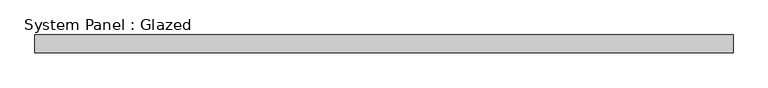
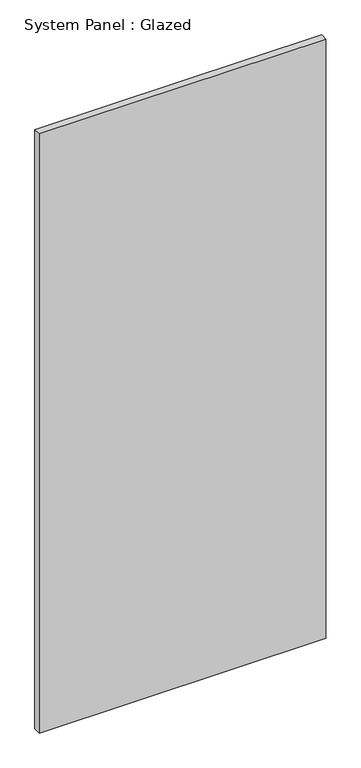
"""IFC4 building model written with IfcOpenShell, lengths in millimetres: plate geometry, System Panel : Glazed."""

from ifc_helpers import new_model, si_unit, origin, origin_with_axes, place, context, project, spatial, polyline, outline, extrude, source, transform, mapped, element, save


def system_panel_glazed_d4561187(model_context):
    return source(origin(), model_context, "Body", "SweptSolid", [
        extrude(outline(polyline([(501.65, 19.05), (-501.65, 19.05), (-501.65, 44.45), (501.65, 44.45), (501.65, 19.05)])), origin_with_axes(), (0.0, 0.0, 1.0), 2216.9308081),
    ])


if __name__ == "__main__":
    model = new_model("IFC4")
    model_context = context("Model", 3, world=origin())
    ifc_project = project(units=[si_unit("LENGTHUNIT", "METRE", prefix="MILLI")], contexts=[model_context])
    site = spatial("IfcSite", under=ifc_project)
    building = spatial("IfcBuilding", under=site)
    placement = place(None, origin())
    system_panel_glazed_shape = system_panel_glazed_d4561187(model_context)
    element("IfcPlate", 1, ObjectType="System Panel : Glazed", at=placement, inside=building, context=model_context, shape_type="MappedRepresentation", body=[
        mapped(system_panel_glazed_shape, transform((0.0, 0.0, 0.0), x_axis=(1.0, 0.0, 0.0), y_axis=(0.0, 1.0, 0.0), z_axis=(0.0, 0.0, 1.0))),
    ])
    save(model, "model.ifc")

# Revit data of these elements
# Type "System Panel : Glazed"
#   Construction Type Id = "GSP4R"
#   Analytic Construction = "1/8 in Pilkington single glazing"
#   Visual Light Transmittance = 0.9
#   Solar Heat Gain Coefficient = 0.86
#   Heat Transfer Coefficient (U) = 1.18115 BTU/(h·ft²·°F)
#   Define Thermal Properties by = 1
# Element 1 (IfcPlate, "System Panel : Glazed")
#   Materials on its faces: "Glass"
# Materials
#   "Glass": class "Glass", colour RGB 0 128 192, transparency 0.75, Description = "Soda Lime Glass", Cost = 0
